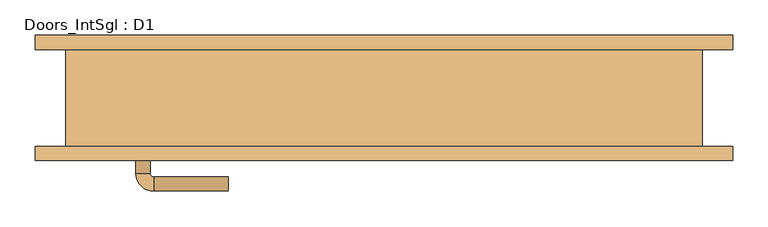
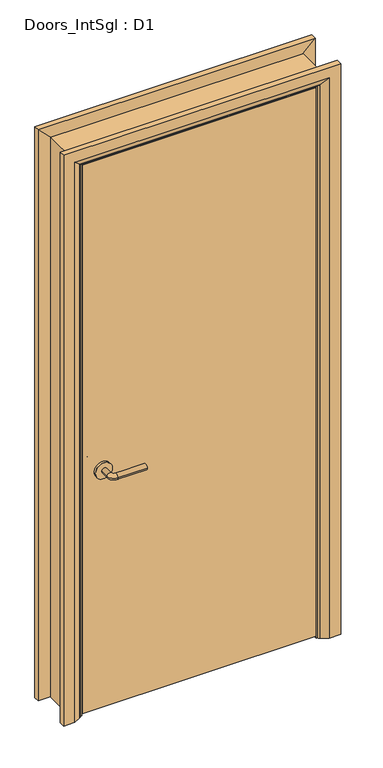
"""IFC4 building model written with IfcOpenShell, lengths in millimetres: door geometry, Doors_IntSgl : D1."""

from ifc_helpers import new_model, si_unit, point, frame, frame_2d, origin, place, context, project, spatial, polyline, circle_curve, ellipse_curve, trimmed, segment, composite_curve, outline, extrude, faceted_brep, source, transform, mapped, element, save
from ifc_brep_helpers import plane_surface, cylinder_surface, revolved_surface, advanced_brep


def doors_intsgl_d1_00c56c0f(model_context):
    return source(origin(), model_context, "Body", "SolidModel", [
        advanced_brep(
        [(-350.2, -22.58, 900.0), (-330.2, -22.58, 900.0), (-350.2, 7.42, 900.0), (-330.2, 7.42, 900.0), (-325.2, 12.42, 900.0), (-325.2, 32.42, 900.0), (-220.2, 32.42, 900.0), (-220.2, 12.42, 900.0)],
        [
            (0, 1, circle_curve(frame((-340.2, -22.58, 900.0), z_axis=(0.0, -1.0, 0.0), x_axis=(1.0, 0.0, 0.0)), 10.0)),
            (1, 0, circle_curve(frame((-340.2, -22.58, 900.0), z_axis=(0.0, -1.0, 0.0), x_axis=(1.0, 0.0, 0.0)), 10.0)),
            (0, 2),
            (2, 3, circle_curve(frame((-340.2, 7.42, 900.0), z_axis=(0.0, -1.0, 0.0), x_axis=(1.0, 0.0, 0.0)), 10.0)),
            (3, 1),
            (3, 2, circle_curve(frame((-340.2, 7.42, 900.0), z_axis=(0.0, -1.0, 0.0), x_axis=(1.0, 0.0, 0.0)), 10.0)),
            (4, 3, circle_curve(frame((-325.2, 7.42, 900.0), z_axis=(0.0, 0.0, 1.0), x_axis=(-1.0, 0.0, 0.0)), 5.0)),
            (2, 5, circle_curve(frame((-325.2, 7.42, 900.0), z_axis=(0.0, 0.0, -1.0), x_axis=(-1.0, 0.0, 0.0)), 25.0)),
            (5, 4, circle_curve(frame((-325.2, 22.42, 900.0), z_axis=(-1.0, 0.0, 0.0), x_axis=(0.0, -1.0, 0.0)), 10.0)),
            (4, 5, circle_curve(frame((-325.2, 22.42, 900.0), z_axis=(-1.0, 0.0, 0.0), x_axis=(0.0, -1.0, 0.0)), 10.0)),
            (6, 7, circle_curve(frame((-220.2, 22.42, 900.0), z_axis=(1.0, 0.0, 0.0), x_axis=(0.0, -1.0, 0.0)), 10.0)),
            (7, 6, circle_curve(frame((-220.2, 22.42, 900.0), z_axis=(1.0, 0.0, 0.0), x_axis=(0.0, -1.0, 0.0)), 10.0)),
            (5, 6),
            (7, 4),
        ],
        [
            plane_surface(frame((-340.2, -22.58, 900.0), z_axis=(0.0, -1.0, 0.0), x_axis=(0.0, 0.0, 1.0))),
            cylinder_surface(frame((-340.2, -22.58, 900.0), z_axis=(0.0, -1.0, 0.0), x_axis=(1.0, 0.0, 0.0)), 10.0),
            revolved_surface(trimmed(ellipse_curve(frame((-340.2, 7.42, 900.0), z_axis=(0.0, -1.0, 0.0), x_axis=(1.0, 0.0, 0.0)), 10.0, 10.0), [point((-350.2, 7.42, 900.0))], [point((-330.2, 7.42, 900.0))], True, "CARTESIAN"), (-325.2, 7.42, 900.0), (0.0, 0.0, -1.0)),
            revolved_surface(trimmed(ellipse_curve(frame((-340.2, 7.42, 900.0), z_axis=(0.0, -1.0, 0.0), x_axis=(1.0, 0.0, 0.0)), 10.0, 10.0), [point((-330.2, 7.42, 900.0))], [point((-350.2, 7.42, 900.0))], True, "CARTESIAN"), (-325.2, 7.42, 900.0), (0.0, 0.0, -1.0)),
            plane_surface(frame((-220.2, 22.42, 900.0), z_axis=(1.0, 0.0, 0.0), x_axis=(0.0, 0.0, 1.0))),
            cylinder_surface(frame((-325.2, 22.42, 900.0), z_axis=(-1.0, 0.0, 0.0), x_axis=(0.0, -1.0, 0.0)), 10.0),
        ],
        [
            (0, [[1, 2]]),
            (1, [[-1, 3, 4, 5]]),
            (1, [[-2, -5, 6, -3]]),
            (2, [[7, -4, 8, 9]]),
            (3, [[-8, -6, -7, 10]]),
            (4, [[11, 12]]),
            (5, [[-9, 13, -12, 14]]),
            (5, [[-10, -14, -11, -13]]),
        ],
    ),
        extrude(outline(composite_curve([segment(trimmed(circle_curve(frame_2d((900.0, -342.7)), 30.0), [point((900.0, -372.7))], [point((900.0, -312.7))], False, "CARTESIAN"), True, "CONTINUOUS"), segment(trimmed(circle_curve(frame_2d((900.0, -342.7)), 30.0), [point((900.0, -312.7))], [point((900.0, -372.7))], False, "CARTESIAN"), True, "CONTINUOUS")], self_intersect=False)), frame((0.0, -30.58, 0.0), z_axis=(0.0, 1.0, 0.0), x_axis=(0.0, 0.0, 1.0)), (0.0, 0.0, 1.0), 8.0),
        advanced_brep(
        [(-350.2, -76.58, 900.0), (-330.2, -76.58, 900.0), (-330.2, -106.58, 900.0), (-350.2, -106.58, 900.0), (-325.2, -111.58, 900.0), (-325.2, -131.58, 900.0), (-220.2, -131.58, 900.0), (-220.2, -111.58, 900.0)],
        [
            (0, 1, circle_curve(frame((-340.2, -76.58, 900.0), z_axis=(0.0, 1.0, 0.0), x_axis=(1.0, 0.0, 0.0)), 10.0)),
            (1, 0, circle_curve(frame((-340.2, -76.58, 900.0), z_axis=(0.0, 1.0, 0.0), x_axis=(1.0, 0.0, 0.0)), 10.0)),
            (1, 2),
            (2, 3, circle_curve(frame((-340.2, -106.58, 900.0), z_axis=(0.0, 1.0, 0.0), x_axis=(1.0, 0.0, 0.0)), 10.0)),
            (3, 0),
            (3, 2, circle_curve(frame((-340.2, -106.58, 900.0), z_axis=(0.0, 1.0, 0.0), x_axis=(1.0, 0.0, 0.0)), 10.0)),
            (4, 5, circle_curve(frame((-325.2, -121.58, 900.0), z_axis=(-1.0, 0.0, 0.0), x_axis=(0.0, 1.0, 0.0)), 10.0)),
            (5, 3, circle_curve(frame((-325.2, -106.58, 900.0), z_axis=(0.0, 0.0, -1.0), x_axis=(-1.0, 0.0, 0.0)), 25.0)),
            (2, 4, circle_curve(frame((-325.2, -106.58, 900.0), z_axis=(0.0, 0.0, 1.0), x_axis=(-1.0, 0.0, 0.0)), 5.0)),
            (5, 4, circle_curve(frame((-325.2, -121.58, 900.0), z_axis=(-1.0, 0.0, 0.0), x_axis=(0.0, 1.0, 0.0)), 10.0)),
            (6, 7, circle_curve(frame((-220.2, -121.58, 900.0), z_axis=(1.0, 0.0, 0.0), x_axis=(0.0, 1.0, 0.0)), 10.0)),
            (7, 6, circle_curve(frame((-220.2, -121.58, 900.0), z_axis=(1.0, 0.0, 0.0), x_axis=(0.0, 1.0, 0.0)), 10.0)),
            (4, 7),
            (6, 5),
        ],
        [
            plane_surface(frame((-340.2, -76.58, 900.0), z_axis=(0.0, 1.0, 0.0), x_axis=(0.0, 0.0, 1.0))),
            cylinder_surface(frame((-340.2, -76.58, 900.0), z_axis=(0.0, 1.0, 0.0), x_axis=(1.0, 0.0, 0.0)), 10.0),
            revolved_surface(trimmed(ellipse_curve(frame((-340.2, -106.58, 900.0), z_axis=(0.0, -1.0, 0.0), x_axis=(1.0, 0.0, 0.0)), 10.0, 10.0), [point((-350.2, -106.58, 900.0))], [point((-330.2, -106.58, 900.0))], True, "CARTESIAN"), (-325.2, -106.58, 900.0), (0.0, 0.0, -1.0)),
            revolved_surface(trimmed(ellipse_curve(frame((-340.2, -106.58, 900.0), z_axis=(0.0, -1.0, 0.0), x_axis=(1.0, 0.0, 0.0)), 10.0, 10.0), [point((-330.2, -106.58, 900.0))], [point((-350.2, -106.58, 900.0))], True, "CARTESIAN"), (-325.2, -106.58, 900.0), (0.0, 0.0, -1.0)),
            plane_surface(frame((-220.2, -121.58, 900.0), z_axis=(1.0, 0.0, 0.0), x_axis=(0.0, 0.0, 1.0))),
            cylinder_surface(frame((-325.2, -121.58, 900.0), z_axis=(-1.0, 0.0, 0.0), x_axis=(0.0, 1.0, 0.0)), 10.0),
        ],
        [
            (0, [[1, 2]]),
            (1, [[3, 4, 5, -2]]),
            (1, [[-5, 6, -3, -1]]),
            (2, [[7, 8, -4, 9]]),
            (3, [[10, -9, -6, -8]]),
            (4, [[11, 12]]),
            (5, [[13, -11, 14, -7]]),
            (5, [[-14, -12, -13, -10]]),
        ],
    ),
        extrude(outline(composite_curve([segment(trimmed(circle_curve(frame_2d((900.0, -342.7)), 30.0), [point((900.0, -372.7))], [point((900.0, -312.7))], False, "CARTESIAN"), True, "CONTINUOUS"), segment(trimmed(circle_curve(frame_2d((900.0, -342.7)), 30.0), [point((900.0, -312.7))], [point((900.0, -372.7))], False, "CARTESIAN"), True, "CONTINUOUS")], self_intersect=False)), frame((0.0, -76.58, 0.0), z_axis=(0.0, 1.0, 0.0), x_axis=(0.0, 0.0, 1.0)), (0.0, 0.0, 1.0), 8.0),
        extrude(outline(polyline([(415.2, -30.58), (415.2, -68.58), (-415.2, -68.58), (-415.2, -30.58), (415.2, -30.58)])), frame((0.0, 0.0, 8.0), z_axis=(0.0, 0.0, 1.0), x_axis=(1.0, 0.0, 0.0)), (0.0, 0.0, 1.0), 2060.0),
        advanced_brep(
        [(492.2, -88.58, 0.0), (452.2, -88.58, 0.0), (426.2, -74.58, 0.0), (422.2, -68.58, 0.0), (492.2, -68.58, 0.0), (492.2, -68.58, 2145.0), (492.2, -88.58, 2145.0), (422.2, -68.58, 2075.0), (-422.2, -68.58, 2075.0), (-422.2, -68.58, 0.0), (-492.2, -68.58, 0.0), (-492.2, -68.58, 2145.0), (426.2, -74.58, 2079.0), (452.2, -88.58, 2105.0), (-492.2, -88.58, 2145.0), (-492.2, -88.58, 0.0), (-452.2, -88.58, 0.0), (-452.2, -88.58, 2105.0), (-426.2, -74.58, 0.0), (-426.2, -74.58, 2079.0)],
        [
            (0, 1),
            (1, 2),
            (2, 3, circle_curve(frame((430.2, -67.58, 0.0), z_axis=(0.0, 0.0, -1.0), x_axis=(1.0, 0.0, 0.0)), 8.0622577)),
            (3, 4),
            (4, 0),
            (4, 5),
            (5, 6),
            (6, 0),
            (3, 7),
            (7, 8),
            (8, 9),
            (9, 10),
            (10, 11),
            (11, 5),
            (2, 12),
            (12, 7, ellipse_curve(frame((430.2, -67.58, 2083.0), z_axis=(0.7071067811865475, 0.0, -0.7071067811865475), x_axis=(-0.7071067811865474, 0.0, -0.7071067811865476)), 11.4017543, 8.0622577)),
            (1, 13),
            (13, 12),
            (6, 14),
            (14, 15),
            (15, 16),
            (16, 17),
            (17, 13),
            (10, 15),
            (14, 11),
            (9, 18, circle_curve(frame((-430.2, -67.58, 0.0), z_axis=(0.0, 0.0, -1.0), x_axis=(-1.0, 0.0, 0.0)), 8.0622577)),
            (18, 16),
            (19, 18),
            (8, 19, ellipse_curve(frame((-430.2, -67.58, 2083.0), z_axis=(-0.7071067811865475, 0.0, -0.7071067811865475), x_axis=(-0.7071067811865474, 0.0, 0.7071067811865476)), 11.4017543, 8.0622577)),
            (19, 17),
            (12, 19),
        ],
        [
            plane_surface(frame((422.2, -68.58, 0.0), z_axis=(0.0, 0.0, -1.0), x_axis=(0.0, 1.0, 0.0))),
            plane_surface(frame((492.2, -88.58, 0.0), z_axis=(1.0, 0.0, 0.0), x_axis=(0.0, 0.0, 1.0))),
            plane_surface(frame((492.2, -68.58, 0.0), z_axis=(0.0, 1.0, 0.0), x_axis=(0.0, 0.0, 1.0))),
            cylinder_surface(frame((430.2, -67.58, 0.0), z_axis=(0.0, 0.0, -1.0), x_axis=(1.0, 0.0, 0.0)), 8.0622577),
            plane_surface(frame((426.2, -74.58, 0.0), z_axis=(-0.4740998230350126, -0.880471099922178, 0.0), x_axis=(0.0, 0.0, 1.0))),
            plane_surface(frame((452.2, -88.58, 0.0), z_axis=(0.0, -1.0, 0.0), x_axis=(0.0, 0.0, 1.0))),
            plane_surface(frame((-492.2, -88.58, 2145.0), z_axis=(-1.0, 0.0, 0.0), x_axis=(0.0, 0.0, -1.0))),
            plane_surface(frame((-422.2, -68.58, 0.0), z_axis=(0.0, 0.0, -1.0), x_axis=(0.0, 1.0, 0.0))),
            cylinder_surface(frame((-430.2, -67.58, 2075.0), z_axis=(0.0, 0.0, 1.0), x_axis=(-1.0, 0.0, 0.0)), 8.0622577),
            plane_surface(frame((-426.2, -74.58, 2079.0), z_axis=(0.47409982303501824, -0.8804710999221749, 0.0), x_axis=(0.0, 0.0, -1.0))),
            plane_surface(frame((492.2, -88.58, 2145.0), z_axis=(0.0, 0.0, 1.0), x_axis=(-1.0, 0.0, 0.0))),
            cylinder_surface(frame((422.2, -67.58, 2083.0), z_axis=(1.0, 0.0, 0.0), x_axis=(0.0, 0.0, 1.0)), 8.0622577),
            plane_surface(frame((426.2, -74.58, 2079.0), z_axis=(0.0, -0.8804710999221764, -0.4740998230350154), x_axis=(-1.0, 0.0, 0.0))),
        ],
        [
            (0, [[1, 2, 3, 4, 5]]),
            (1, [[6, 7, 8, -5]]),
            (2, [[9, 10, 11, 12, 13, 14, -6, -4]]),
            (3, [[15, 16, -9, -3]]),
            (4, [[17, 18, -15, -2]]),
            (5, [[-8, 19, 20, 21, 22, 23, -17, -1]]),
            (6, [[-13, 24, -20, 25]]),
            (7, [[-24, -12, 26, 27, -21]]),
            (8, [[28, -26, -11, 29]]),
            (9, [[-22, -27, -28, 30]]),
            (10, [[-14, -25, -19, -7]]),
            (11, [[31, -29, -10, -16]]),
            (12, [[-23, -30, -31, -18]]),
        ],
    ),
        extrude(outline(polyline([(0.0, -398.2), (2051.0, -398.2), (2051.0, 398.2), (0.0, 398.2), (0.0, 417.2), (2070.0, 417.2), (2070.0, -417.2), (0.0, -417.2), (0.0, -398.2)])), frame((0.0, -28.58, 0.0), z_axis=(0.0, 1.0, 0.0), x_axis=(0.0, 0.0, 1.0)), (0.0, 0.0, 1.0), 32.0),
        advanced_brep(
        [(-492.2, 88.58, 0.0), (-452.2, 88.58, 0.0), (-426.2, 74.58, 0.0), (-422.2, 68.58, 0.0), (-492.2, 68.58, 0.0), (-492.2, 68.58, 2145.0), (-492.2, 88.58, 2145.0), (-422.2, 68.58, 2075.0), (-426.2, 74.58, 2079.0), (-452.2, 88.58, 2105.0), (492.2, 88.58, 0.0), (492.2, 68.58, 0.0), (422.2, 68.58, 0.0), (426.2, 74.58, 0.0), (452.2, 88.58, 0.0), (492.2, 88.58, 2145.0), (452.2, 88.58, 2105.0), (426.2, 74.58, 2079.0), (422.2, 68.58, 2075.0), (492.2, 68.58, 2145.0)],
        [
            (0, 1),
            (1, 2),
            (2, 3, circle_curve(frame((-430.2, 67.58, 0.0), z_axis=(0.0, 0.0, -1.0), x_axis=(-1.0, 0.0, 0.0)), 8.0622577)),
            (3, 4),
            (4, 0),
            (4, 5),
            (5, 6),
            (6, 0),
            (3, 7),
            (7, 5),
            (2, 8),
            (8, 7, ellipse_curve(frame((-430.2, 67.58, 2083.0), z_axis=(-0.7071067811865475, 0.0, -0.7071067811865475), x_axis=(0.7071067811865474, 0.0, -0.7071067811865476)), 11.4017543, 8.0622577)),
            (1, 9),
            (9, 8),
            (6, 9),
            (10, 11),
            (11, 12),
            (12, 13, circle_curve(frame((430.2, 67.58, 0.0), z_axis=(0.0, 0.0, -1.0), x_axis=(1.0, 0.0, 0.0)), 8.0622577)),
            (13, 14),
            (14, 10),
            (15, 10),
            (14, 16),
            (16, 15),
            (13, 17),
            (17, 16),
            (12, 18),
            (18, 17, ellipse_curve(frame((430.2, 67.58, 2083.0), z_axis=(0.7071067811865475, 0.0, -0.7071067811865475), x_axis=(0.7071067811865474, 0.0, 0.7071067811865476)), 11.4017543, 8.0622577)),
            (11, 19),
            (19, 18),
            (15, 19),
            (5, 19),
            (15, 6),
            (7, 18),
            (8, 17),
            (9, 16),
        ],
        [
            plane_surface(frame((-422.2, 141.3810989, 0.0), z_axis=(0.0, 0.0, -1.0), x_axis=(1.0, 0.0, 0.0))),
            plane_surface(frame((-492.2, 88.58, 0.0), z_axis=(-1.0, 0.0, 0.0), x_axis=(0.0, 0.0, 1.0))),
            plane_surface(frame((-492.2, 68.58, 0.0), z_axis=(0.0, -1.0, 0.0), x_axis=(0.0, 0.0, 1.0))),
            cylinder_surface(frame((-430.2, 67.58, 0.0), z_axis=(0.0, 0.0, -1.0), x_axis=(-1.0, 0.0, 0.0)), 8.0622577),
            plane_surface(frame((-426.2, 74.58, 0.0), z_axis=(0.4740998230350183, 0.8804710999221749, 0.0), x_axis=(0.0, 0.0, 1.0))),
            plane_surface(frame((-452.2, 88.58, 0.0), z_axis=(0.0, 1.0, 0.0), x_axis=(0.0, 0.0, 1.0))),
            plane_surface(frame((422.2, 141.3810989, 0.0), z_axis=(0.0, 0.0, -1.0), x_axis=(-1.0, 0.0, 0.0))),
            plane_surface(frame((452.2, 88.58, 2105.0), z_axis=(0.0, 1.0, 0.0), x_axis=(0.0, 0.0, -1.0))),
            plane_surface(frame((426.2, 74.58, 2079.0), z_axis=(-0.4740998230350183, 0.8804710999221749, 0.0), x_axis=(0.0, 0.0, -1.0))),
            cylinder_surface(frame((430.2, 67.58, 2075.0), z_axis=(0.0, 0.0, 1.0), x_axis=(1.0, 0.0, 0.0)), 8.0622577),
            plane_surface(frame((492.2, 68.58, 2145.0), z_axis=(0.0, -1.0, 0.0), x_axis=(0.0, 0.0, -1.0))),
            plane_surface(frame((492.2, 88.58, 2145.0), z_axis=(1.0, 0.0, 0.0), x_axis=(0.0, 0.0, -1.0))),
            plane_surface(frame((-492.2, 88.58, 2145.0), z_axis=(0.0, 0.0, 1.0), x_axis=(1.0, 0.0, 0.0))),
            plane_surface(frame((-492.2, 68.58, 2145.0), z_axis=(0.0, -1.0, 0.0), x_axis=(1.0, 0.0, 0.0))),
            cylinder_surface(frame((-422.2, 67.58, 2083.0), z_axis=(-1.0, 0.0, 0.0), x_axis=(0.0, 0.0, 1.0)), 8.0622577),
            plane_surface(frame((-426.2, 74.58, 2079.0), z_axis=(0.0, 0.8804710999221749, -0.4740998230350183), x_axis=(1.0, 0.0, 0.0))),
            plane_surface(frame((-452.2, 88.58, 2105.0), z_axis=(0.0, 1.0, 0.0), x_axis=(1.0, 0.0, 0.0))),
        ],
        [
            (0, [[1, 2, 3, 4, 5]]),
            (1, [[6, 7, 8, -5]]),
            (2, [[9, 10, -6, -4]]),
            (3, [[11, 12, -9, -3]]),
            (4, [[13, 14, -11, -2]]),
            (5, [[-8, 15, -13, -1]]),
            (6, [[16, 17, 18, 19, 20]]),
            (7, [[21, -20, 22, 23]]),
            (8, [[-22, -19, 24, 25]]),
            (9, [[-24, -18, 26, 27]]),
            (10, [[-26, -17, 28, 29]]),
            (11, [[-28, -16, -21, 30]]),
            (12, [[31, -30, 32, -7]]),
            (13, [[33, -29, -31, -10]]),
            (14, [[34, -27, -33, -12]]),
            (15, [[35, -25, -34, -14]]),
            (16, [[-32, -23, -35, -15]]),
        ],
    ),
        faceted_brep([(-417.2, -68.58, 0.0), (-449.2, -68.58, 0.0), (-449.2, 68.58, 0.0), (-417.2, 68.58, 0.0), (-417.2, 68.58, 2070.0), (-417.2, -68.58, 2070.0), (-449.2, 68.58, 2102.0), (-449.2, -68.58, 2102.0), (417.2, -68.58, 0.0), (417.2, 68.58, 0.0), (449.2, 68.58, 0.0), (449.2, -68.58, 0.0), (417.2, -68.58, 2070.0), (449.2, -68.58, 2102.0), (449.2, 68.58, 2102.0), (417.2, 68.58, 2070.0)], [[[0, 1, 2, 3]], [[3, 4, 5, 0]], [[2, 6, 4, 3]], [[1, 7, 6, 2]], [[0, 5, 7, 1]], [[8, 9, 10, 11]], [[12, 8, 11, 13]], [[13, 11, 10, 14]], [[14, 10, 9, 15]], [[15, 9, 8, 12]], [[4, 15, 12, 5]], [[6, 14, 15, 4]], [[7, 13, 14, 6]], [[5, 12, 13, 7]]]),
    ])


if __name__ == "__main__":
    model = new_model("IFC4")
    model_context = context("Model", 3, world=origin())
    ifc_project = project(units=[si_unit("LENGTHUNIT", "METRE", prefix="MILLI")], contexts=[model_context])
    site = spatial("IfcSite", under=ifc_project)
    building = spatial("IfcBuilding", under=site)
    placement = place(None, origin())
    doors_intsgl_d1_shape = doors_intsgl_d1_00c56c0f(model_context)
    element("IfcDoor", 1, ObjectType="Doors_IntSgl : D1", at=placement, inside=building, context=model_context, shape_type="MappedRepresentation", body=[
        mapped(doors_intsgl_d1_shape, transform((0.0, 0.0, 0.0), x_axis=(1.0, 0.0, 0.0), y_axis=(0.0, 1.0, 0.0), z_axis=(0.0, 0.0, 1.0))),
    ])
    save(model, "model.ifc")

# Revit data of these elements
# Type "Doors_IntSgl : D1"
#   Type Mark = "46"
#   Type Comments = "Internal Single"
#   Operation = "SingleSwingRight"
#   Manufacturer = "Revit"
#   Keynote = "L20"
#   Description = "Internal Single Door"
#   Analytic Construction = "Metal"
#   UnderCut = 0.026247 ft
#   Tolerance = 0.006562 ft
#   Thickness = 0.124672 ft
#   Thermal Resistance (R) = 0.270117 (m²·K)/W
#   Structural Tolerance = 0.026247 ft
#   StopDepth = 0.104987 ft
#   Stop Thickness = 0.062336 ft
#   Rough Width = 3.0 ft
#   Rough Height = 6.922572 ft
#   Height to Top Lock Rail = 3.28084 ft
#   Heat Transfer Coefficient (U) = 3.7021 W/(m²·K)
#   Handle Z Distance = 2.952756 ft
#   Handle X Distance = 0.246063 ft
#   Frame Thickness = 0.104987 ft
#   Door Panel Width = 2.724409 ft
#   Door Panel Thickness = 0.124672 ft
#   Door Panel Offset = 0.0 ft
#   Height = 6.922572 ft
#   Width = 3.0 ft
#   Door Panel Height = 6.75853 ft
#   Architrave Setback = 0.016404 ft
#   Vis - Ironmongery = yes
#   Material Ironmongery = Door - Handle
#   Material Frame = Door - Frame/Mullion (1)
#   Material Door = Door - Panel
#   Material Architrave = Door - Architrave
#   Visual Light Transmittance = 0
#   Solar Heat Gain Coefficient = 0
#   Function = (empty or 0)
#   Wall Closure = (empty or 0)
# Element 1 (IfcDoor, "Doors_IntSgl : D1")
#   Materials on its faces: "Door - Architrave", "Door - Handle", "Door - Frame/Mullion (1)", "Door - Panel"
# Materials
#   "Door - Handle": colour RGB 0 0 0, transparency 0, Keynote = "P21", Cost = 0
#   "Door - Frame/Mullion (1)": class "Wood", colour RGB 212 179 113, transparency 0, Keynote = "L20", Cost = 0
#   "Door - Panel": class "Wood", colour RGB 210 159 95, transparency 0, Keynote = "L20", Cost = 0
#   "Door - Architrave": class "Wood", colour RGB 154 90 5, transparency 0, Keynote = "P20", Cost = 0
